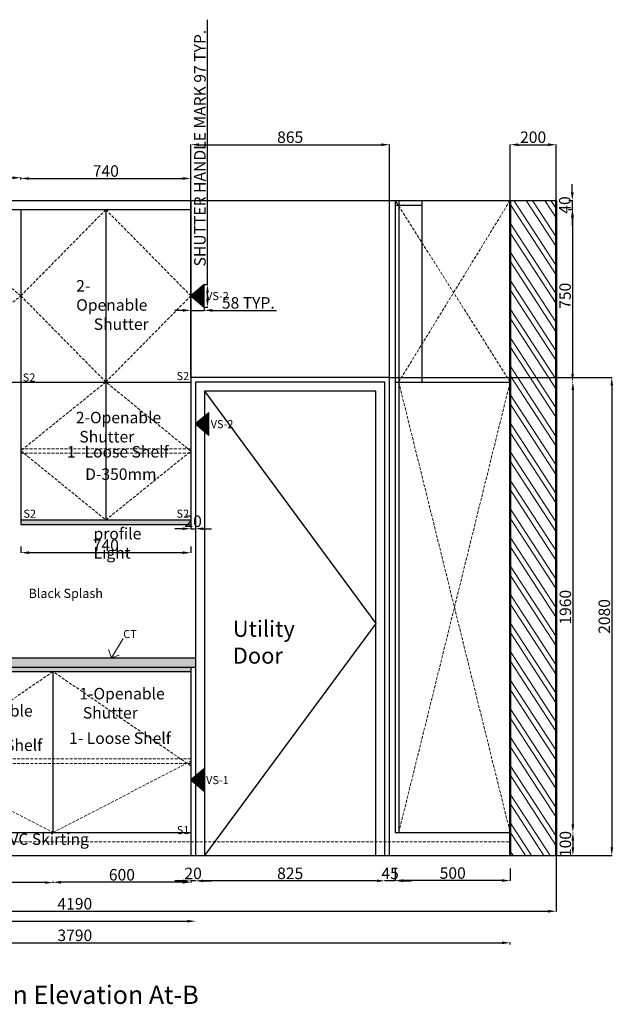
# Model space of a CAD drawing. Units: millimetres. Extents: x 407065 to 421840, y 1168257 to 1177792.
# Tile 17 of 17: x 419256 to 421840, y 1173419 to 1177702. Entities that reach past the tile are written whole.
import ezdxf

# ---------------------------------------------------------------- set-up
doc = ezdxf.new("R2010")
doc.units = ezdxf.units.MM
doc.linetypes.add('DASHED', pattern=[19.05, 12.7, -6.35])
for name, color, linetype, lineweight in [('A-ANNO-DIMS', 6, 'Continuous', 18), ('A-ANNO-SYMB', 6, 'Continuous', 18), ('A-ANNO-TEXT', 30, 'Continuous', 18), ('A-DOOR', 4, 'Continuous', 25), ('A-FURN', 3, 'Continuous', 25), ('A-FURN-HIDN', 7, 'DASHED', 18), ('A-FURN-PATT', 252, 'Continuous', 13), ('A-WALL', 7, 'Continuous', 50), ('A-WALL-PATT', 8, 'Continuous', 13)]:
    doc.layers.add(name, color=color, linetype=linetype, lineweight=lineweight)
doc.styles.get("Standard").update_dxf_attribs({"font": 'arial.ttf'})
doc.dimstyles.new('ISO-25', dxfattribs={"dimtxt": 50, "dimasz": 35, "dimexe": 1.25, "dimexo": 0.625, "dimtad": 1, "dimdec": 1, "dimtxsty": 'Standard', "dimcen": 35, "dimadec": 0, "dimazin": 0, "dimtfac": 1, "dimtdec": 1, "dimtmove": 0, "dimatfit": 3, "dimfxl": 1, "dimarcsym": 0})

# ---------------------------------------------------------------- blocks, each defined once
blk = doc.blocks.new('*D86')
at = {"layer": 'A-ANNO-DIMS', "color": 0, "lineweight": -2, "transparency": 16777216}
for p, q in [((418331.3, 1177007.2), (418331.3, 1177016.1)), ((418366.3, 1177014.9), (419226.3, 1177014.9)), ((419261.3, 1177007.2), (419261.3, 1177016.1))]:
    blk.add_line(p, q, dxfattribs=at)
at = {"layer": 'A-ANNO-DIMS', "color": 0, "transparency": 16777216}
for points in [[(418366.3, 1177020.7), (418366.3, 1177009), (418331.3, 1177014.9)], [(419226.3, 1177020.7), (419226.3, 1177009), (419261.3, 1177014.9)]]:
    blk.add_solid(points, dxfattribs=at)
at = {"layer": 'Defpoints', "color": 0, "transparency": 16777216}
for p in [(419261.3, 1177014.9), (418331.3, 1177006.6), (419261.3, 1177006.6)]:
    blk.add_point(p, dxfattribs=at)
at = {"layer": 'A-ANNO-DIMS', "color": 0, "transparency": 16777216, "insert": (418796.3, 1177041), "char_height": 50, "attachment_point": 5}
blk.add_mtext('930', dxfattribs=at)
blk = doc.blocks.new('*D87')
at = {"layer": 'A-ANNO-DIMS', "color": 0, "lineweight": -2, "transparency": 16777216}
for p, q in [((419261.3, 1177015.5), (419261.3, 1177010.4)), ((420001.3, 1177015.5), (420001.3, 1177010.4)), ((419296.3, 1177011.7), (419966.3, 1177011.7))]:
    blk.add_line(p, q, dxfattribs=at)
at = {"layer": 'A-ANNO-DIMS', "color": 0, "transparency": 16777216}
for points in [[(419296.3, 1177017.5), (419296.3, 1177005.8), (419261.3, 1177011.7)], [(419966.3, 1177017.5), (419966.3, 1177005.8), (420001.3, 1177011.7)]]:
    blk.add_solid(points, dxfattribs=at)
at = {"layer": 'Defpoints', "color": 0, "transparency": 16777216}
for p in [(419261.3, 1177016.1), (420001.3, 1177016.1), (420001.3, 1177011.7)]:
    blk.add_point(p, dxfattribs=at)
at = {"layer": 'A-ANNO-DIMS', "color": 0, "transparency": 16777216, "insert": (419631.3, 1177037.8), "char_height": 50, "attachment_point": 5}
blk.add_mtext('740', dxfattribs=at)
blk = doc.blocks.new('*D88')
at = {"layer": 'A-ANNO-DIMS', "color": 0, "lineweight": -2, "transparency": 16777216}
for p, q in [((421661.8, 1176951.2), (421661.8, 1176986.2)), ((421646.8, 1176916.2), (421663.1, 1176916.2)), ((421661.8, 1176916.2), (421661.8, 1176876.2)), ((421646, 1176876.2), (421663.1, 1176876.2)), ((421661.8, 1176841.2), (421661.8, 1176806.2))]:
    blk.add_line(p, q, dxfattribs=at)
at = {"layer": 'A-ANNO-DIMS', "color": 0, "transparency": 16777216}
for points in [[(421656, 1176951.2), (421667.7, 1176951.2), (421661.8, 1176916.2)], [(421656, 1176841.2), (421667.7, 1176841.2), (421661.8, 1176876.2)]]:
    blk.add_solid(points, dxfattribs=at)
at = {"layer": 'Defpoints', "color": 0, "transparency": 16777216}
for p in [(421646.2, 1176916.2), (421645.3, 1176876.2), (421661.8, 1176876.2)]:
    blk.add_point(p, dxfattribs=at)
at = {"layer": 'A-ANNO-DIMS', "color": 0, "transparency": 16777216, "insert": (421635.7, 1176896.2), "char_height": 50, "attachment_point": 5, "rotation": 90}
blk.add_mtext('40', dxfattribs=at)
blk = doc.blocks.new('*D89')
at = {"layer": 'A-ANNO-DIMS', "color": 0, "lineweight": -2, "transparency": 16777216}
for p, q in [((421662.5, 1176876.2), (421664.3, 1176876.2)), ((421663.1, 1176841.2), (421663.1, 1176161.2)), ((421662.5, 1176126.2), (421664.3, 1176126.2))]:
    blk.add_line(p, q, dxfattribs=at)
at = {"layer": 'A-ANNO-DIMS', "color": 0, "transparency": 16777216}
for points in [[(421657.3, 1176841.2), (421668.9, 1176841.2), (421663.1, 1176876.2)], [(421657.3, 1176161.2), (421668.9, 1176161.2), (421663.1, 1176126.2)]]:
    blk.add_solid(points, dxfattribs=at)
at = {"layer": 'Defpoints', "color": 0, "transparency": 16777216}
for p in [(421661.8, 1176876.2), (421661.8, 1176126.2), (421663.1, 1176126.2)]:
    blk.add_point(p, dxfattribs=at)
at = {"layer": 'A-ANNO-DIMS', "color": 0, "transparency": 16777216, "insert": (421636.9, 1176501.2), "char_height": 50, "attachment_point": 5, "rotation": 90}
blk.add_mtext('750', dxfattribs=at)
blk = doc.blocks.new('*D90')
at = {"layer": 'A-ANNO-DIMS', "color": 0, "lineweight": -2, "transparency": 16777216}
for p, q in [((421665, 1176126.2), (421665.6, 1176126.2)), ((421664.3, 1176091.2), (421664.3, 1174201.2)), ((421665, 1174166.2), (421665.6, 1174166.2))]:
    blk.add_line(p, q, dxfattribs=at)
at = {"layer": 'A-ANNO-DIMS', "color": 0, "transparency": 16777216}
for points in [[(421658.5, 1176091.2), (421670.2, 1176091.2), (421664.3, 1176126.2)], [(421658.5, 1174201.2), (421670.2, 1174201.2), (421664.3, 1174166.2)]]:
    blk.add_solid(points, dxfattribs=at)
at = {"layer": 'Defpoints', "color": 0, "transparency": 16777216}
for p in [(421664.3, 1176126.2), (421664.3, 1174166.2), (421664.3, 1174166.2)]:
    blk.add_point(p, dxfattribs=at)
at = {"layer": 'A-ANNO-DIMS', "color": 0, "transparency": 16777216, "insert": (421638.2, 1175146.2), "char_height": 50, "attachment_point": 5, "rotation": 90}
blk.add_mtext('1960', dxfattribs=at)
blk = doc.blocks.new('*D91')
at = {"layer": 'A-ANNO-DIMS', "color": 0, "lineweight": -2, "transparency": 16777216}
for p, q in [((421663.7, 1174166.2), (421665.6, 1174166.2)), ((421664.3, 1174131.2), (421664.3, 1174101.2)), ((421663.7, 1174066.2), (421665.6, 1174066.2))]:
    blk.add_line(p, q, dxfattribs=at)
at = {"layer": 'A-ANNO-DIMS', "color": 0, "transparency": 16777216}
for points in [[(421658.5, 1174131.2), (421670.2, 1174131.2), (421664.3, 1174166.2)], [(421658.5, 1174101.2), (421670.2, 1174101.2), (421664.3, 1174066.2)]]:
    blk.add_solid(points, dxfattribs=at)
at = {"layer": 'Defpoints', "color": 0, "transparency": 16777216}
for p in [(421663.1, 1174166.2), (421663.1, 1174066.2), (421664.3, 1174066.2)]:
    blk.add_point(p, dxfattribs=at)
at = {"layer": 'A-ANNO-DIMS', "color": 0, "transparency": 16777216, "insert": (421638.2, 1174116.2), "char_height": 50, "attachment_point": 5, "rotation": 90}
blk.add_mtext('100', dxfattribs=at)
blk = doc.blocks.new('*D92')
at = {"layer": 'A-ANNO-DIMS', "color": 0, "lineweight": -2, "transparency": 16777216}
for p, q in [((420891.3, 1174010.1), (420891.3, 1173956)), ((421391.3, 1174010.1), (421391.3, 1173956)), ((421356.3, 1173957.2), (420926.3, 1173957.2))]:
    blk.add_line(p, q, dxfattribs=at)
at = {"layer": 'A-ANNO-DIMS', "color": 0, "transparency": 16777216}
for points in [[(420926.3, 1173963.1), (420926.3, 1173951.4), (420891.3, 1173957.2)], [(421356.3, 1173963.1), (421356.3, 1173951.4), (421391.3, 1173957.2)]]:
    blk.add_solid(points, dxfattribs=at)
at = {"layer": 'Defpoints', "color": 0, "transparency": 16777216}
for p in [(420891.3, 1174010.8), (421391.3, 1174010.8), (420891.3, 1173957.2)]:
    blk.add_point(p, dxfattribs=at)
at = {"layer": 'A-ANNO-DIMS', "color": 0, "transparency": 16777216, "insert": (421141.3, 1173983.4), "char_height": 50, "attachment_point": 5}
blk.add_mtext('500', dxfattribs=at)
blk = doc.blocks.new('*D93')
at = {"layer": 'A-ANNO-DIMS', "color": 0, "lineweight": -2, "transparency": 16777216}
for p, q in [((420811.3, 1173956), (420776.3, 1173956)), ((420846.3, 1173956.6), (420846.3, 1173957.2)), ((420891.3, 1173956), (420846.3, 1173956)), ((420891.3, 1173956.6), (420891.3, 1173957.2)), ((420926.3, 1173956), (420961.3, 1173956))]:
    blk.add_line(p, q, dxfattribs=at)
at = {"layer": 'A-ANNO-DIMS', "color": 0, "transparency": 16777216}
for points in [[(420811.3, 1173961.8), (420811.3, 1173950.1), (420846.3, 1173956)], [(420926.3, 1173961.8), (420926.3, 1173950.1), (420891.3, 1173956)]]:
    blk.add_solid(points, dxfattribs=at)
at = {"layer": 'Defpoints', "color": 0, "transparency": 16777216}
for p in [(420846.3, 1173956), (420846.3, 1173956), (420891.3, 1173956)]:
    blk.add_point(p, dxfattribs=at)
at = {"layer": 'A-ANNO-DIMS', "color": 0, "transparency": 16777216, "insert": (420868.8, 1173982), "char_height": 50, "attachment_point": 5}
blk.add_mtext('45', dxfattribs=at)
blk = doc.blocks.new('*D94')
at = {"layer": 'A-ANNO-DIMS', "color": 0, "lineweight": -2, "transparency": 16777216}
for p, q in [((420021.3, 1173956.6), (420021.3, 1173957.2)), ((420811.3, 1173956), (420056.3, 1173956)), ((420846.3, 1173956.6), (420846.3, 1173957.2))]:
    blk.add_line(p, q, dxfattribs=at)
at = {"layer": 'A-ANNO-DIMS', "color": 0, "transparency": 16777216}
for points in [[(420056.3, 1173961.8), (420056.3, 1173950.1), (420021.3, 1173956)], [(420811.3, 1173961.8), (420811.3, 1173950.1), (420846.3, 1173956)]]:
    blk.add_solid(points, dxfattribs=at)
at = {"layer": 'Defpoints', "color": 0, "transparency": 16777216}
for p in [(420021.3, 1173956), (420021.3, 1173956), (420846.3, 1173956)]:
    blk.add_point(p, dxfattribs=at)
at = {"layer": 'A-ANNO-DIMS', "color": 0, "transparency": 16777216, "insert": (420433.8, 1173982.1), "char_height": 50, "attachment_point": 5}
blk.add_mtext('825', dxfattribs=at)
blk = doc.blocks.new('*D95')
at = {"layer": 'A-ANNO-DIMS', "color": 0, "lineweight": -2, "transparency": 16777216}
for p, q in [((419966.3, 1173955.6), (419931.3, 1173955.6)), ((420021.3, 1173955.6), (420001.3, 1173955.6)), ((420001.3, 1173955.3), (420001.3, 1173954.3)), ((420021.3, 1173955.3), (420021.3, 1173954.3)), ((420056.3, 1173955.6), (420091.3, 1173955.6))]:
    blk.add_line(p, q, dxfattribs=at)
at = {"layer": 'A-ANNO-DIMS', "color": 0, "transparency": 16777216}
for points in [[(419966.3, 1173961.4), (419966.3, 1173949.8), (420001.3, 1173955.6)], [(420056.3, 1173961.4), (420056.3, 1173949.8), (420021.3, 1173955.6)]]:
    blk.add_solid(points, dxfattribs=at)
at = {"layer": 'Defpoints', "color": 0, "transparency": 16777216}
for p in [(420001.3, 1173956), (420001.3, 1173955.6), (420021.3, 1173956)]:
    blk.add_point(p, dxfattribs=at)
at = {"layer": 'A-ANNO-DIMS', "color": 0, "transparency": 16777216, "insert": (420011.3, 1173981.7), "char_height": 50, "attachment_point": 5}
blk.add_mtext('20', dxfattribs=at)
blk = doc.blocks.new('*D96')
at = {"layer": 'A-ANNO-DIMS', "color": 0, "lineweight": -2, "transparency": 16777216}
for p, q in [((419401.3, 1173953.7), (419401.3, 1173948.5)), ((419966.3, 1173949.8), (419436.3, 1173949.8)), ((420001.3, 1173953.7), (420001.3, 1173948.5))]:
    blk.add_line(p, q, dxfattribs=at)
at = {"layer": 'A-ANNO-DIMS', "color": 0, "transparency": 16777216}
for points in [[(419436.3, 1173955.6), (419436.3, 1173943.9), (419401.3, 1173949.8)], [(419966.3, 1173955.6), (419966.3, 1173943.9), (420001.3, 1173949.8)]]:
    blk.add_solid(points, dxfattribs=at)
at = {"layer": 'Defpoints', "color": 0, "transparency": 16777216}
for p in [(419401.3, 1173954.3), (419401.3, 1173949.8), (420001.3, 1173954.3)]:
    blk.add_point(p, dxfattribs=at)
at = {"layer": 'A-ANNO-DIMS', "color": 0, "transparency": 16777216, "insert": (419701.3, 1173975.9), "char_height": 50, "attachment_point": 5}
blk.add_mtext('600', dxfattribs=at)
blk = doc.blocks.new('*D97')
at = {"layer": 'A-ANNO-DIMS', "color": 0, "lineweight": -2, "transparency": 16777216}
for p, q in [((418801.3, 1173953.7), (418801.3, 1173947.3)), ((419366.3, 1173948.5), (418836.3, 1173948.5)), ((419401.3, 1173953.7), (419401.3, 1173947.3))]:
    blk.add_line(p, q, dxfattribs=at)
at = {"layer": 'A-ANNO-DIMS', "color": 0, "transparency": 16777216}
for points in [[(418836.3, 1173954.3), (418836.3, 1173942.7), (418801.3, 1173948.5)], [(419366.3, 1173954.3), (419366.3, 1173942.7), (419401.3, 1173948.5)]]:
    blk.add_solid(points, dxfattribs=at)
at = {"layer": 'Defpoints', "color": 0, "transparency": 16777216}
for p in [(418801.3, 1173954.3), (418801.3, 1173948.5), (419401.3, 1173954.3)]:
    blk.add_point(p, dxfattribs=at)
at = {"layer": 'A-ANNO-DIMS', "color": 0, "transparency": 16777216, "insert": (419101.3, 1173974.7), "char_height": 50, "attachment_point": 5}
blk.add_mtext('600', dxfattribs=at)
blk = doc.blocks.new('*D102')
at = {"layer": 'A-ANNO-DIMS', "color": 0, "lineweight": -2, "transparency": 16777216}
for p, q in [((417601.3, 1173779.7), (417601.3, 1173779.1)), ((417636.3, 1173780.4), (419986.3, 1173780.4)), ((420021.3, 1173779.7), (420021.3, 1173779.1))]:
    blk.add_line(p, q, dxfattribs=at)
at = {"layer": 'A-ANNO-DIMS', "color": 0, "transparency": 16777216}
for points in [[(417636.3, 1173786.2), (417636.3, 1173774.5), (417601.3, 1173780.4)], [(419986.3, 1173786.2), (419986.3, 1173774.5), (420021.3, 1173780.4)]]:
    blk.add_solid(points, dxfattribs=at)
at = {"layer": 'Defpoints', "color": 0, "transparency": 16777216}
for p in [(417601.3, 1173780.4), (420021.3, 1173780.4), (420021.3, 1173780.4)]:
    blk.add_point(p, dxfattribs=at)
at = {"layer": 'A-ANNO-DIMS', "color": 0, "transparency": 16777216, "insert": (418811.3, 1173806.5), "char_height": 50, "attachment_point": 5}
blk.add_mtext('2420', dxfattribs=at)
blk = doc.blocks.new('*D103')
at = {"layer": 'A-ANNO-DIMS', "color": 0, "lineweight": -2, "transparency": 16777216}
for p, q in [((417601.3, 1173679.4), (417601.3, 1173687.7)), ((417636.3, 1173686.5), (421356.3, 1173686.5)), ((421391.3, 1173679.4), (421391.3, 1173687.7))]:
    blk.add_line(p, q, dxfattribs=at)
at = {"layer": 'A-ANNO-DIMS', "color": 0, "transparency": 16777216}
for points in [[(417636.3, 1173692.3), (417636.3, 1173680.6), (417601.3, 1173686.5)], [(421356.3, 1173692.3), (421356.3, 1173680.6), (421391.3, 1173686.5)]]:
    blk.add_solid(points, dxfattribs=at)
at = {"layer": 'Defpoints', "color": 0, "transparency": 16777216}
for p in [(417601.3, 1173678.8), (421391.3, 1173686.5), (421391.3, 1173678.8)]:
    blk.add_point(p, dxfattribs=at)
at = {"layer": 'A-ANNO-DIMS', "color": 0, "transparency": 16777216, "insert": (419496.3, 1173712.6), "char_height": 50, "attachment_point": 5}
blk.add_mtext('3790', dxfattribs=at)
blk = doc.blocks.new('*D116')
at = {"layer": 'A-ANNO-DIMS', "color": 0, "lineweight": -2, "transparency": 16777216}
for p, q in [((419966.3, 1175487.9), (419931.3, 1175487.9)), ((420001.3, 1175505.5), (420001.3, 1175486.6)), ((420001.3, 1175487.9), (420021.3, 1175487.9)), ((420021.3, 1175505.5), (420021.3, 1175486.6)), ((420056.3, 1175487.9), (420091.3, 1175487.9))]:
    blk.add_line(p, q, dxfattribs=at)
at = {"layer": 'A-ANNO-DIMS', "color": 0, "transparency": 16777216}
for points in [[(419966.3, 1175493.7), (419966.3, 1175482.1), (420001.3, 1175487.9)], [(420056.3, 1175493.7), (420056.3, 1175482.1), (420021.3, 1175487.9)]]:
    blk.add_solid(points, dxfattribs=at)
at = {"layer": 'Defpoints', "color": 0, "transparency": 16777216}
for p in [(420001.3, 1175506.2), (420021.3, 1175506.2), (420021.3, 1175487.9)]:
    blk.add_point(p, dxfattribs=at)
at = {"layer": 'A-ANNO-DIMS', "color": 0, "transparency": 16777216, "insert": (420011.3, 1175514), "char_height": 50, "attachment_point": 5}
blk.add_mtext('20', dxfattribs=at)
blk = doc.blocks.new('*D117')
at = {"layer": 'A-ANNO-DIMS', "color": 0, "lineweight": -2, "transparency": 16777216}
for p, q in [((419261.3, 1175411.1), (419261.3, 1175382.4)), ((420001.3, 1175411.1), (420001.3, 1175382.4)), ((419966.3, 1175383.7), (419296.3, 1175383.7))]:
    blk.add_line(p, q, dxfattribs=at)
at = {"layer": 'A-ANNO-DIMS', "color": 0, "transparency": 16777216}
for points in [[(419296.3, 1175389.5), (419296.3, 1175377.9), (419261.3, 1175383.7)], [(419966.3, 1175389.5), (419966.3, 1175377.9), (420001.3, 1175383.7)]]:
    blk.add_solid(points, dxfattribs=at)
at = {"layer": 'Defpoints', "color": 0, "transparency": 16777216}
for p in [(419261.3, 1175411.8), (420001.3, 1175411.8), (419261.3, 1175383.7)]:
    blk.add_point(p, dxfattribs=at)
at = {"layer": 'A-ANNO-DIMS', "color": 0, "transparency": 16777216, "insert": (419631.3, 1175409.8), "char_height": 50, "attachment_point": 5}
blk.add_mtext('740', dxfattribs=at)
blk = doc.blocks.new('SHUTTER-HANDLE-MARK')
h = blk.add_hatch()
h.set_pattern_fill('ANSI32', color=256, scale=0.08)
h.set_pattern_definition([(45, (-3404.92366, -221.627), (-0.53881536726, 0.53881536726), []), (45, (-3404.56445, -221.627), (-0.53881536726, 0.53881536726), [])])
h.paths.add_polyline_path([(420059.2, 1176549.9), (420001.3, 1176501.2), (420059.2, 1176452.5)])
h = blk.add_hatch(color=256)
h.dxf.hatch_style = 1
h.paths.add_polyline_path([(420059.2, 1176549.9), (420001.3, 1176501.2), (420059.2, 1176452.5)])
blk = doc.blocks.new('*D163')
at = {"layer": 'A-ANNO-DIMS', "color": 0, "lineweight": -2, "transparency": 16777216}
for p, q in [((420073.8, 1176549.9), (420073.8, 1177702.5)), ((420059.8, 1176549.9), (420075.1, 1176549.9)), ((420073.8, 1176487.5), (420073.8, 1176514.9)), ((420059.8, 1176452.5), (420075.1, 1176452.5))]:
    blk.add_line(p, q, dxfattribs=at)
at = {"layer": 'A-ANNO-DIMS', "color": 0, "transparency": 16777216}
for points in [[(420068, 1176514.9), (420079.6, 1176514.9), (420073.8, 1176549.9)], [(420068, 1176487.5), (420079.6, 1176487.5), (420073.8, 1176452.5)]]:
    blk.add_solid(points, dxfattribs=at)
at = {"layer": 'Defpoints', "color": 0, "transparency": 16777216}
for p in [(420059.2, 1176549.9), (420073.8, 1176549.9), (420059.2, 1176452.5)]:
    blk.add_point(p, dxfattribs=at)
at = {"layer": 'A-ANNO-DIMS', "color": 0, "transparency": 16777216, "insert": (420047.3, 1177143.7), "char_height": 50, "attachment_point": 5, "rotation": 90}
blk.add_mtext('SHUTTER HANDLE MARK 97 TYP.', dxfattribs=at)
blk = doc.blocks.new('*D164')
at = {"layer": 'A-ANNO-DIMS', "color": 0, "lineweight": -2, "transparency": 16777216}
for p, q in [((419966.3, 1176437.9), (419931.3, 1176437.9)), ((420001.3, 1176451.9), (420001.3, 1176436.6)), ((420001.3, 1176437.9), (420059.2, 1176437.9)), ((420059.2, 1176451.9), (420059.2, 1176436.6)), ((420094.2, 1176437.9), (420373.8, 1176437.9))]:
    blk.add_line(p, q, dxfattribs=at)
at = {"layer": 'A-ANNO-DIMS', "color": 0, "transparency": 16777216}
for points in [[(419966.3, 1176443.7), (419966.3, 1176432), (420001.3, 1176437.9)], [(420094.2, 1176443.7), (420094.2, 1176432), (420059.2, 1176437.9)]]:
    blk.add_solid(points, dxfattribs=at)
at = {"layer": 'Defpoints', "color": 0, "transparency": 16777216}
for p in [(420001.3, 1176452.5), (420059.2, 1176452.5), (420059.2, 1176437.9)]:
    blk.add_point(p, dxfattribs=at)
at = {"layer": 'A-ANNO-DIMS', "color": 0, "transparency": 16777216, "insert": (420251.5, 1176464), "char_height": 50, "attachment_point": 5}
blk.add_mtext('58 TYP.', dxfattribs=at)
blk = doc.blocks.new('*D200')
at = {"layer": 'A-ANNO-DIMS', "color": 0, "lineweight": -2, "transparency": 16777216}
for p, q in [((417401.3, 1174065.5), (417401.3, 1173822.4)), ((421591.3, 1174065.5), (421591.3, 1173822.4)), ((417436.3, 1173823.7), (421556.3, 1173823.7))]:
    blk.add_line(p, q, dxfattribs=at)
at = {"layer": 'A-ANNO-DIMS', "color": 0, "transparency": 16777216}
for points in [[(417436.3, 1173829.5), (417436.3, 1173817.8), (417401.3, 1173823.7)], [(421556.3, 1173829.5), (421556.3, 1173817.8), (421591.3, 1173823.7)]]:
    blk.add_solid(points, dxfattribs=at)
at = {"layer": 'Defpoints', "color": 0, "transparency": 16777216}
for p in [(417401.3, 1174066.2), (421591.3, 1174066.2), (421591.3, 1173823.7)]:
    blk.add_point(p, dxfattribs=at)
at = {"layer": 'A-ANNO-DIMS', "color": 0, "transparency": 16777216, "insert": (419496.3, 1173849.8), "char_height": 50, "attachment_point": 5}
blk.add_mtext('4190', dxfattribs=at)
blk = doc.blocks.new('*D202')
at = {"layer": 'A-ANNO-DIMS', "color": 0, "lineweight": -2, "transparency": 16777216}
for p, q in [((421391.3, 1176916.8), (421391.3, 1177159.9)), ((421426.3, 1177158.7), (421556.3, 1177158.7)), ((421591.3, 1176916.8), (421591.3, 1177159.9))]:
    blk.add_line(p, q, dxfattribs=at)
at = {"layer": 'A-ANNO-DIMS', "color": 0, "transparency": 16777216}
for points in [[(421426.3, 1177164.5), (421426.3, 1177152.8), (421391.3, 1177158.7)], [(421556.3, 1177164.5), (421556.3, 1177152.8), (421591.3, 1177158.7)]]:
    blk.add_solid(points, dxfattribs=at)
at = {"layer": 'Defpoints', "color": 0, "transparency": 16777216}
for p in [(421591.3, 1177158.7), (421391.3, 1176916.2), (421591.3, 1176916.2)]:
    blk.add_point(p, dxfattribs=at)
at = {"layer": 'A-ANNO-DIMS', "color": 0, "transparency": 16777216, "insert": (421491.3, 1177184.8), "char_height": 50, "attachment_point": 5}
blk.add_mtext('200', dxfattribs=at)
blk = doc.blocks.new('*D206')
at = {"layer": 'A-ANNO-DIMS', "color": 0, "lineweight": -2, "transparency": 16777216}
for p, q in [((420001.3, 1176146.8), (420001.3, 1177159.9)), ((420036.3, 1177158.7), (420831.3, 1177158.7)), ((420866.3, 1176146.8), (420866.3, 1177159.9))]:
    blk.add_line(p, q, dxfattribs=at)
at = {"layer": 'A-ANNO-DIMS', "color": 0, "transparency": 16777216}
for points in [[(420036.3, 1177164.5), (420036.3, 1177152.8), (420001.3, 1177158.7)], [(420831.3, 1177164.5), (420831.3, 1177152.8), (420866.3, 1177158.7)]]:
    blk.add_solid(points, dxfattribs=at)
at = {"layer": 'Defpoints', "color": 0, "transparency": 16777216}
for p in [(420866.3, 1177158.7), (420001.3, 1176146.2), (420866.3, 1176146.2)]:
    blk.add_point(p, dxfattribs=at)
at = {"layer": 'A-ANNO-DIMS', "color": 0, "transparency": 16777216, "insert": (420433.8, 1177184.8), "char_height": 50, "attachment_point": 5}
blk.add_mtext('865', dxfattribs=at)
blk = doc.blocks.new('*D207')
at = {"layer": 'A-ANNO-DIMS', "color": 0, "lineweight": -2, "transparency": 16777216}
for p, q in [((420866.9, 1176146.2), (421835, 1176146.2)), ((421833.8, 1176111.2), (421833.8, 1174101.2)), ((421391.9, 1174066.2), (421835, 1174066.2))]:
    blk.add_line(p, q, dxfattribs=at)
at = {"layer": 'A-ANNO-DIMS', "color": 0, "transparency": 16777216}
for points in [[(421827.9, 1176111.2), (421839.6, 1176111.2), (421833.8, 1176146.2)], [(421827.9, 1174101.2), (421839.6, 1174101.2), (421833.8, 1174066.2)]]:
    blk.add_solid(points, dxfattribs=at)
at = {"layer": 'Defpoints', "color": 0, "transparency": 16777216}
for p in [(420866.3, 1176146.2), (421391.3, 1174066.2), (421833.8, 1174066.2)]:
    blk.add_point(p, dxfattribs=at)
at = {"layer": 'A-ANNO-DIMS', "color": 0, "transparency": 16777216, "insert": (421807.6, 1175106.2), "char_height": 50, "attachment_point": 5, "rotation": 90}
blk.add_mtext('2080', dxfattribs=at)

msp = doc.modelspace()

# ---------------------------------------------------------------- hatches: boundary and pattern name
at = {"layer": 'A-FURN-PATT'}
h = msp.add_hatch(color=256, dxfattribs=at)
h.dxf.hatch_style = 1
h.paths.add_polyline_path([(420001.277, 1175526.1682), (419261.277, 1175526.1682), (419261.277, 1175506.1682), (420001.277, 1175506.1682)])
h = msp.add_hatch(dxfattribs=at)
h.set_pattern_fill('AR-CONC', color=256, scale=0.08)
h.set_pattern_definition([(50, (-3404.924, -221.627), (14.57477352, -1.27512684), [1.524, -16.764]), (355, (-3404.924, -221.627), (-2.81947371, 15.28454762), [1.2192, -13.41124673]), (100.4514447, (-3403.709, -221.733), (11.75529977, 14.00942015), [1.2952007, -14.24721957]), (46.1842, (-3404.924, -217.563), (21.68632327, -3.36338623), [2.286, -25.146]), (96.6355576, (-3403.116, -217.843), (18.99233072, 19.79408997), [1.94280185, -21.37084865]), (351.1841512, (-3404.924, -217.563), (18.99233073, 19.79408997), [1.82879737, -20.11677855]), (21, (-3402.892, -218.579), (12.1291513, -8.18121585), [1.524, -16.764]), (326, (-3402.892, -218.579), (4.94416227, 14.73503729), [1.2192, -13.4112]), (71.451445, (-3401.881, -219.261), (17.07331354, 6.55382151), [1.2952007, -14.247195]), (37.5, (-3404.9237, -221.627), (0.24708826, 6.76440311), [0, -13.24864, 0, -13.6144, 0, -13.462]), (7.5, (-3404.924, -221.627), (5.345573, 8.014445985), [0, -7.76224, 0, -12.94384, 0, -5.1308]), (327.5, (-3409.455, -221.627), (10.847247613, -0.45829952), [0, -5.08, 0, -15.8496, 0, -21.0312]), (317.5, (-3411.487, -221.627), (11.85033451, 2.03411928), [0, -6.604, 0, -10.52576, 0, -14.9352])])
h.paths.add_polyline_path([(420021.277, 1174926.1682), (417601.277, 1174926.1682), (417601.277, 1174886.1682), (420021.277, 1174886.1682)])
h = msp.add_hatch(color=256, dxfattribs=at)
h.dxf.hatch_style = 1
h.paths.add_polyline_path([(420001.277, 1174886.1682), (418181.277, 1174886.1682), (418181.277, 1174866.1682), (420001.277, 1174866.1682)])
at = {"layer": 'A-WALL-PATT'}
h = msp.add_hatch(dxfattribs=at)
h.set_pattern_fill('ANSI32', color=256, scale=7.1, angle=78)
h.set_pattern_definition([(123, (-3404.924, -221.63), (-56.717194, -36.8325763), []), (123, (-3398.295, -190.444), (-56.717194, -36.8325763), [])])
h.paths.add_polyline_path([(421591.277, 1176916.1682), (421391.277, 1176916.1682), (421391.277, 1174066.1682), (421591.277, 1174066.1682)])

# ---------------------------------------------------------------- linework, layer by layer
at = {"layer": 'A-ANNO-SYMB'}
for p, q in [((419707.1331, 1175010.863), (419655.3391, 1174926.1682)), ((419655.3391, 1174926.1682), (419643.2066, 1174962.7938)), ((419655.3391, 1174926.1682), (419689.9806, 1174937.6435))]:
    msp.add_line(p, q, dxfattribs=at)
at = {"layer": 'A-DOOR'}
for p, q in [((420061.277, 1176086.1682), (420806.277, 1175076.1682)), ((420806.277, 1175076.1682), (420061.277, 1174066.1682))]:
    msp.add_line(p, q, dxfattribs=at)
for points in [[(420806.277, 1174066.1682), (420806.277, 1176086.1682), (420061.277, 1176086.1682), (420061.277, 1174066.1682)], [(420001.277, 1174886.1682), (420001.277, 1174066.1682)]]:
    msp.add_lwpolyline(points, dxfattribs=at)
for points in [[(420079.4172, 1175992.5585), (420021.4941, 1175943.8747), (420079.4172, 1175895.1909)], [(420059.2, 1174443.9176), (420001.277, 1174395.2338), (420059.2, 1174346.55)]]:
    msp.add_lwpolyline(points, close=True, dxfattribs=at)
at = {"layer": 'A-FURN'}
for p, q in [((417401.277, 1176916.1682), (421591.277, 1176916.1682)), ((420001.277, 1176916.1682), (420001.277, 1175506.1682)), ((420891.277, 1176916.1682), (420891.277, 1174166.1682)), ((420891.277, 1176896.1682), (421006.277, 1176896.1682)), ((420906.277, 1176916.1682), (420906.277, 1174166.1682)), ((421006.277, 1176916.1682), (421006.277, 1176126.1682)), ((417841.277, 1176876.1682), (420001.277, 1176876.1682)), ((419261.277, 1176876.1682), (419261.277, 1175506.1682)), ((419631.277, 1176876.1682), (419631.277, 1175526.1682)), ((417601.277, 1176126.1682), (420001.277, 1176126.1682)), ((420891.277, 1176146.1682), (421006.277, 1176146.1682)), ((420891.277, 1176126.1682), (421391.277, 1176126.1682)), ((419261.277, 1175526.1682), (420001.277, 1175526.1682)), ((419261.277, 1175506.1682), (420001.277, 1175506.1682)), ((417601.277, 1174926.1682), (420021.277, 1174926.1682)), ((417601.277, 1174886.1682), (420021.277, 1174886.1682)), ((418181.277, 1174866.1682), (420001.277, 1174866.1682)), ((417601.277, 1174166.1682), (420001.277, 1174166.1682)), ((420891.277, 1174166.1682), (421391.277, 1174166.1682)), ((417401.277, 1174066.1682), (421591.277, 1174066.1682))]:
    msp.add_line(p, q, dxfattribs=at)
msp.add_lwpolyline([(420059.2, 1176549.852), (420001.277, 1176501.1682), (420059.2, 1176452.4845)], close=True, dxfattribs=at)
for points in [[(420866.277, 1174066.1682), (420866.277, 1176146.1682), (420001.277, 1176146.1682)], [(420846.277, 1174066.1682), (420846.277, 1176126.1682), (420021.277, 1176126.1682), (420021.277, 1174066.1682)], [(419401.277, 1174866.1682), (419401.277, 1174166.1682)]]:
    msp.add_lwpolyline(points, dxfattribs=at)
at = {"layer": 'A-FURN-HIDN'}
for p, q in [((421391.277, 1176126.1682), (420891.277, 1176916.1682)), ((421391.277, 1176916.1682), (420906.277, 1176126.1682)), ((419261.277, 1176501.1682), (418796.277, 1176876.1682)), ((419631.277, 1176876.1682), (419261.277, 1176501.1682)), ((420001.277, 1176501.1682), (419631.277, 1176876.1682)), ((418796.277, 1176126.1682), (419261.277, 1176501.1682)), ((419261.277, 1176501.1682), (419631.277, 1176126.1682)), ((419631.277, 1176126.1682), (420001.277, 1176501.1682)), ((419631.277, 1176126.1682), (419261.277, 1175826.8781)), ((420001.277, 1175824.9568), (419631.277, 1176126.1682)), ((420906.277, 1176126.1682), (421391.277, 1174166.1682)), ((420906.277, 1174166.1682), (421391.277, 1176126.1682)), ((419261.277, 1175836.1682), (420001.277, 1175836.1682)), ((419261.277, 1175826.8781), (419631.277, 1175526.1682)), ((419261.277, 1175816.1682), (420001.277, 1175816.1682)), ((419631.277, 1175526.1682), (420001.277, 1175824.9568)), ((419401.277, 1174866.1682), (418801.277, 1174456.1682)), ((420001.277, 1174456.1682), (419401.277, 1174866.1682)), ((420001.277, 1174486.1682), (417601.277, 1174486.1682)), ((420001.277, 1174466.1682), (417601.277, 1174466.1682)), ((418801.277, 1174476.1682), (419401.277, 1174166.1682)), ((419401.277, 1174166.1682), (420001.277, 1174476.1682)), ((417601.277, 1174126.1682), (421391.277, 1174126.1682))]:
    msp.add_line(p, q, dxfattribs=at)
at = {"layer": 'A-WALL'}
for p, q in [((421391.277, 1176916.1682), (421391.277, 1174066.1682)), ((421591.277, 1176916.1682), (421591.277, 1174066.1682))]:
    msp.add_line(p, q, dxfattribs=at)

# ---------------------------------------------------------------- block references
at = {"layer": 'A-FURN'}
for p in [(0, 0), (20.2171, -557.2935), (0, -2105.9344)]:
    msp.add_blockref('SHUTTER-HANDLE-MARK', p, dxfattribs=at)

# ---------------------------------------------------------------- texts
at = {"layer": 'A-ANNO-TEXT', "attachment_point": 1}
for s, width, insert, char_height in [('2- Openable\\P     Shutter', 382.409863, (419502.3117, 1176569.5979), 50), ('VS-2', 382.409863, (420067.6631, 1176517.6678), 35), ('S2', 382.409863, (419269.601, 1176163.3149), 35), ('S2', 382.409863, (419939.0543, 1176169.6109), 35), ('     2-Openable\\P      Shutter', 520.083559, (419424.3303, 1175996.5312), 50), ('VS-2', 382.409863, (420087.8803, 1175960.3743), 35), ('1- Loose Shelf', 475.855052, (419461.7405, 1175847.6043), 50), ('D-350mm', 382.409863, (419541.366, 1175750.2865), 50), ('S2', 382.409863, (419272.6808, 1175570.7235), 35), ('S2', 382.409863, (419938.9246, 1175570.7235), 35), ('profile Light', 382.409863, (419577.8412, 1175491.4345), 50), ('Black Splash', 382.409863, (419295.1964, 1175226.582), 40), ('Utility Door', 507.457786, (420183.8621, 1175087.6783), 70), ('CT', 382.409863, (419707.1331, 1175047.0568), 35), ('     1-Openable\\P      Shutter', 520.083559, (419439.6788, 1174795.3806), 50), ('     1-Openable\\P      Shutter', 520.083559, (418864.8173, 1174720.715), 50), ('\\pxt7;1- Loose Shelf', 487.590713, (418911.573, 1174571.1227), 50), ('\\pxt7;1- Loose Shelf', 487.590713, (419471.4065, 1174601.6335), 50), ('VS-1', 382.409863, (420067.6631, 1174411.7333), 35), ('S1', 382.409863, (419940.387, 1174194.2824), 35), ('    PVC Skirting', 640.76562, (419106.9011, 1174162.362), 50), ('Kitchen Elevation At-B', 1357.183536, (418901.2019, 1173500.2608), 80)]:
    msp.add_mtext_dynamic_manual_height_columns(s, width=width, gutter_width=12.5, heights=[0], dxfattribs=dict(at, insert=insert, char_height=char_height))

# ---------------------------------------------------------------- dimensions: what is measured, and where the dimension line sits
at = {"layer": 'A-ANNO-DIMS'}
dim = msp.add_linear_dim(base=(420073.8052, 1176549.852), p1=(420059.2, 1176452.4845), p2=(420059.2, 1176549.852), angle=90, text='SHUTTER HANDLE MARK <> TYP.', dimstyle='ISO-25', override={"dimdec": 0, "dimrnd": 0, "dimzin": 0, "dimlunit": 2}, dxfattribs=at)
dim.commit()
dim.dimension.update_dxf_attribs({"geometry": '*D163', "text_midpoint": (420047.3275, 1177143.6626)})
for base, p1, p2, override, picture, middle in [((420866.277, 1177158.6682), (420001.277, 1176146.1682), (420866.277, 1176146.1682), {"dimdec": 0, "dimlfac": 1, "dimrnd": 0, "dimzin": 0, "dimdsep": 46, "dimlunit": 2}, '*D206', (420433.777, 1177184.8219)), ((421591.277, 1177158.6682), (421391.277, 1176916.1682), (421591.277, 1176916.1682), {"dimdec": 0, "dimlfac": 1, "dimrnd": 0, "dimzin": 0, "dimdsep": 46, "dimlunit": 2}, '*D202', (421491.277, 1177184.8219)), ((419261.277, 1177014.8769), (418331.277, 1177006.5676), (419261.277, 1177006.5676), {"dimclrd": 0, "dimclre": 0, "dimclrt": 0}, '*D86', (418796.277, 1177041.0476)), ((420001.277, 1177011.6598), (419261.277, 1177016.1269), (420001.277, 1177016.1269), {"dimclrd": 0, "dimclre": 0, "dimclrt": 0}, '*D87', (419631.277, 1177037.8134)), ((419261.277, 1175383.6954), (420001.277, 1175411.7644), (419261.277, 1175411.7644), {"dimclrd": 0, "dimclre": 0, "dimclrt": 0}, '*D117', (419631.277, 1175409.849)), ((421591.277, 1173823.6682), (417401.277, 1174066.1682), (421591.277, 1174066.1682), {"dimdec": 0, "dimlfac": 1, "dimrnd": 0, "dimzin": 0, "dimdsep": 46, "dimlunit": 2}, '*D200', (419496.277, 1173849.8219)), ((420021.277, 1173955.9712), (420846.277, 1173955.9712), (420021.277, 1173955.9712), {"dimclrd": 0, "dimclre": 0, "dimclrt": 0}, '*D94', (420433.777, 1173982.1248)), ((420891.277, 1173957.2212), (421391.277, 1174010.7572), (420891.277, 1174010.7572), {"dimclrd": 0, "dimclre": 0, "dimclrt": 0}, '*D92', (421141.277, 1173983.3748)), ((418801.277, 1173948.513), (419401.277, 1173954.3463), (418801.277, 1173954.3463), {"dimclrd": 0, "dimclre": 0, "dimclrt": 0}, '*D97', (419101.277, 1173974.6666)), ((419401.277, 1173949.763), (420001.277, 1173954.3463), (419401.277, 1173954.3463), {"dimclrd": 0, "dimclre": 0, "dimclrt": 0}, '*D96', (419701.277, 1173975.9166)), ((420021.277, 1173780.3642), (417601.277, 1173780.3668), (420021.277, 1173780.3668), {"dimclrd": 0, "dimclre": 0, "dimclrt": 0}, '*D102', (418811.277, 1173806.5178)), ((421391.277, 1173686.4606), (417601.277, 1173678.7822), (421391.277, 1173678.7822), {"dimclrd": 0, "dimclre": 0, "dimclrt": 0}, '*D103', (419496.277, 1173712.6313))]:
    dim = msp.add_linear_dim(base=base, p1=p1, p2=p2, dimstyle='ISO-25', override=override, dxfattribs=at)
    dim.commit()
    dim.dimension.update_dxf_attribs({"geometry": picture, "text_midpoint": middle})
for base, p1, p2, picture, middle in [((421661.8385, 1176876.1682), (421646.2128, 1176916.1682), (421645.3447, 1176876.1682), '*D88', (421661.8385, 1176896.1682)), ((421664.3385, 1174066.1682), (421663.0885, 1174166.1682), (421663.0885, 1174066.1682), '*D91', (421664.3385, 1174116.1682))]:
    dim = msp.add_linear_dim(base=base, p1=p1, p2=p2, angle=90, dimstyle='ISO-25', override={"dimclrd": 0, "dimclre": 0, "dimclrt": 0}, dxfattribs=at)
    dim.commit()
    dim.dimension.update_dxf_attribs({"geometry": picture, "text_midpoint": middle, "dimtype": 160})
for base, p1, p2, override, picture, middle in [((421663.0885, 1176126.1682), (421661.8385, 1176876.1682), (421661.8385, 1176126.1682), {"dimclrd": 0, "dimclre": 0, "dimclrt": 0}, '*D89', (421636.9348, 1176501.1682)), ((421833.777, 1174066.1682), (420866.277, 1176146.1682), (421391.277, 1174066.1682), {"dimdec": 0, "dimlfac": 1, "dimrnd": 0, "dimzin": 0, "dimdsep": 46, "dimlunit": 2}, '*D207', (421807.6234, 1175106.1682)), ((421664.3385, 1174166.1682), (421664.3385, 1176126.1682), (421664.3385, 1174166.1682), {"dimclrd": 0, "dimclre": 0, "dimclrt": 0}, '*D90', (421638.1848, 1175146.1682))]:
    dim = msp.add_linear_dim(base=base, p1=p1, p2=p2, angle=90, dimstyle='ISO-25', override=override, dxfattribs=at)
    dim.commit()
    dim.dimension.update_dxf_attribs({"geometry": picture, "text_midpoint": middle})
dim = msp.add_linear_dim(base=(420059.2, 1176437.8793), p1=(420001.277, 1176452.4845), p2=(420059.2, 1176452.4845), text='<> TYP.', dimstyle='ISO-25', override={"dimdec": 0, "dimrnd": 0, "dimzin": 0, "dimlunit": 2}, dxfattribs=at)
dim.commit()
dim.dimension.update_dxf_attribs({"geometry": '*D164', "text_midpoint": (420251.5167, 1176464.033)})
for base, p1, p2, picture, middle in [((420021.277, 1175487.8834), (420001.277, 1175506.1682), (420021.277, 1175506.1682), '*D116', (420011.277, 1175487.8834)), ((420846.277, 1173955.9712), (420891.277, 1173955.9712), (420846.277, 1173955.9712), '*D93', (420868.777, 1173955.9712)), ((420001.277, 1173955.5963), (420021.277, 1173955.9712), (420001.277, 1173955.9712), '*D95', (420011.277, 1173955.5963))]:
    dim = msp.add_linear_dim(base=base, p1=p1, p2=p2, dimstyle='ISO-25', override={"dimclrd": 0, "dimclre": 0, "dimclrt": 0}, dxfattribs=at)
    dim.commit()
    dim.dimension.update_dxf_attribs({"geometry": picture, "text_midpoint": middle, "dimtype": 160})

doc.saveas('drawing.dxf')
